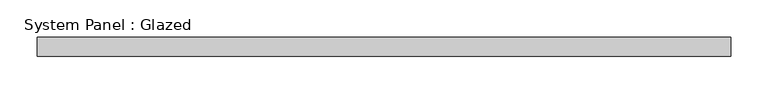
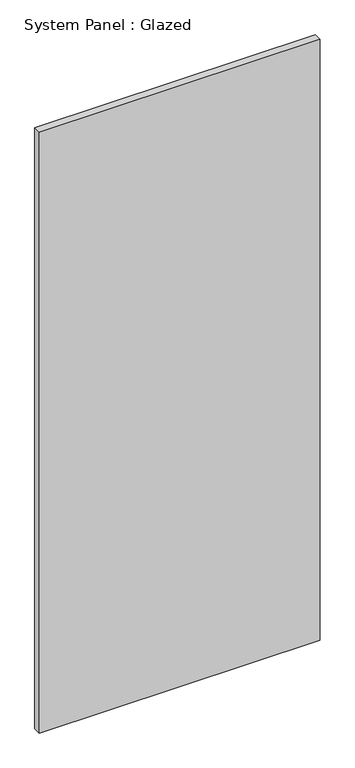
"""IFC4 building model written with IfcOpenShell, lengths in millimetres: plate geometry, System Panel : Glazed."""

from ifc_helpers import new_model, si_unit, origin, origin_with_axes, place, context, project, spatial, polyline, outline, extrude, source, transform, mapped, element, save


def system_panel_glazed_63ec7693(model_context):
    return source(origin(), model_context, "Body", "SweptSolid", [
        extrude(outline(polyline([(463.95, 24.5), (-463.95, 24.5), (-463.95, 49.5), (463.95, 49.5), (463.95, 24.5)])), origin_with_axes(), (0.0, 0.0, 1.0), 2096.7065107),
    ])


if __name__ == "__main__":
    model = new_model("IFC4")
    model_context = context("Model", 3, world=origin())
    ifc_project = project(units=[si_unit("LENGTHUNIT", "METRE", prefix="MILLI")], contexts=[model_context])
    site = spatial("IfcSite", under=ifc_project)
    building = spatial("IfcBuilding", under=site)
    placement = place(None, origin())
    system_panel_glazed_shape = system_panel_glazed_63ec7693(model_context)
    element("IfcPlate", 1, ObjectType="System Panel : Glazed", at=placement, inside=building, context=model_context, shape_type="MappedRepresentation", body=[
        mapped(system_panel_glazed_shape, transform((0.0, 0.0, 0.0), x_axis=(1.0, 0.0, 0.0), y_axis=(0.0, 1.0, 0.0), z_axis=(0.0, 0.0, 1.0))),
    ])
    save(model, "model.ifc")

# Revit data of these elements
# Type "System Panel : Glazed"
#   Keynote = "H11"
#   Construction Type Id = "GSP4R"
#   Analytic Construction = "1/8 in Pilkington single glazing"
#   Visual Light Transmittance = 0.9
#   Solar Heat Gain Coefficient = 0.86
#   Heat Transfer Coefficient (U) = 6.7069 W/(m²·K)
#   Define Thermal Properties by = 1
# Element 1 (IfcPlate, "System Panel : Glazed")
#   Materials on its faces: "Glass"
# Materials
#   "Glass": class "Glass", colour RGB 0 128 192, transparency 0.9, Description = "Soda Lime Glass", Cost = 0
